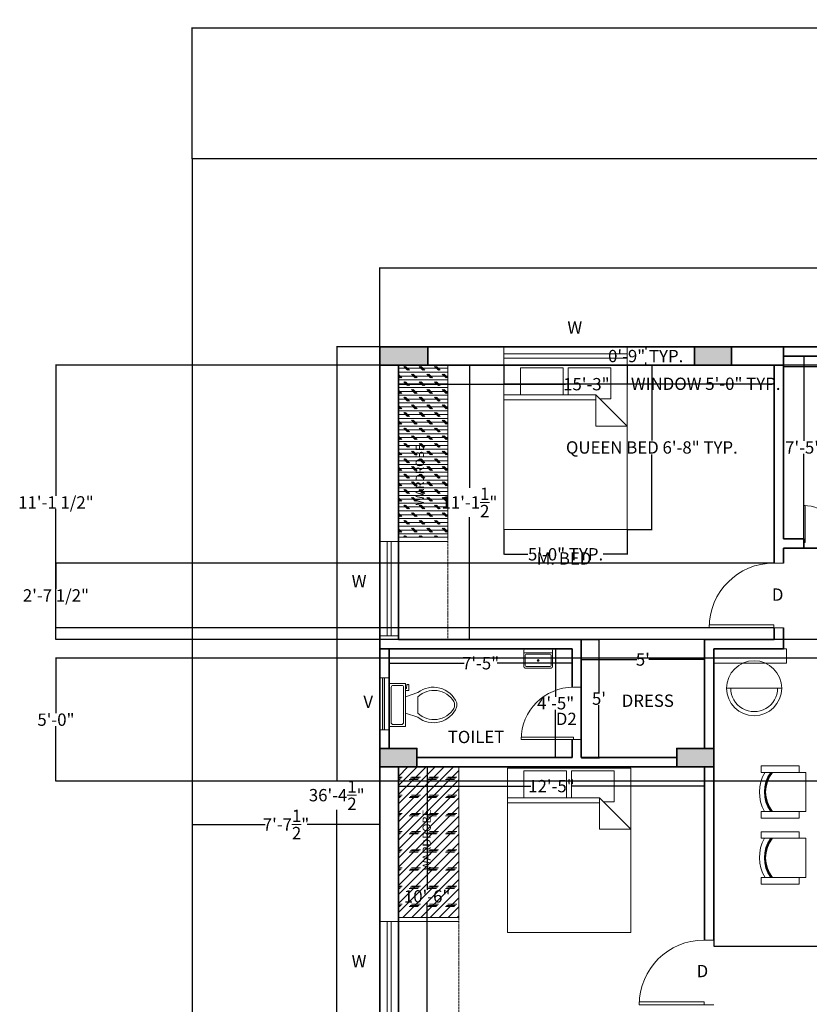
# Model space of a CAD drawing. Units: inches. Extents: x -2181 to 1225, y -80 to 4016.
# Tile 2 of 10: x -77 to 308, y 253 to 732. Entities that reach past the tile are written whole.
import ezdxf

# ---------------------------------------------------------------- set-up
doc = ezdxf.new("R2010")
doc.units = ezdxf.units.IN
doc.header["$MEASUREMENT"] = 0
doc.linetypes.add('ACAD_ISO02W100', pattern=[15, 12, -3])
for name, color, linetype, lineweight in [('A-ANNO-DIMS', 2, 'Continuous', 18), ('A-ANNO-TEXT', 7, 'Continuous', 18), ('A-AREA-IDEN', 7, 'Continuous', 18), ('A-COLS', 7, 'Continuous', 35), ('A-COLS-PATT', 252, 'Continuous', 13), ('A-DOOR', 3, 'Continuous', 18), ('A-FLOR-FIXT', 8, 'Continuous', 18), ('A-FURN', 30, 'Continuous', 18), ('A-GLAZ', 4, 'Continuous', 18), ('A-GLAZ-PATT', 4, 'Continuous', 13), ('A-MILL', 8, 'Continuous', 18), ('A-MILL-OVHD', 8, 'ACAD_ISO02W100', 13), ('A-MILL-PATT', 252, 'Continuous', 13), ('A-WALL', 7, 'Continuous', 35), ('A-WALL-OVHD', 7, 'ACAD_ISO02W100', 18), ('C-PROP', 7, 'Continuous', 30)]:
    doc.layers.add(name, color=color, linetype=linetype, lineweight=lineweight)
doc.styles.get("Standard").update_dxf_attribs({"font": 'arial.ttf'})
doc.dimstyles.get("Standard").update_dxf_attribs({"dimtxt": 6, "dimasz": 0.18, "dimexe": 0.18, "dimexo": 0.0625, "dimgap": 0.09, "dimtad": 0, "dimtih": 1, "dimtoh": 1, "dimdec": 4, "dimzin": 0, "dimdsep": 46, "dimlunit": 4, "dimtxsty": 'Standard', "dimcen": 0.09, "dimadec": 0, "dimazin": 0, "dimtfac": 1, "dimtdec": 4, "dimtofl": 0, "dimtmove": 0, "dimatfit": 3, "dimfxl": 1, "dimtolj": 1, "dimtzin": 0, "dimarcsym": 0})

# ---------------------------------------------------------------- blocks, each defined once
blk = doc.blocks.new('*U2')
for p, q in [((0, 0), (0, -6)), ((40, 0), (40, -6))]:
    blk.add_line(p, q)
blk.add_lwpolyline([(0, 0), (0, 40), (1.75, 40), (1.75, 0)], close=True)
blk.add_arc((0, 0), 40, 0, 90)
blk = doc.blocks.new('*U21')
for p, q in [((9.5, -6), (9.5, -2)), ((-10, -8.5), (-8, -8.5)), ((-10, -9.5), (-10, -8.5)), ((-7, -9.5), (-10, -9.5)), ((-8, -8.5), (-8, -8)), ((-7, -8), (-7, -9.5)), ((-4, -8), (-6, -14)), ((4, -8), (6, -14)), ((4, -14), (-4, -14))]:
    blk.add_line(p, q)
blk.add_lwpolyline([(10.5, -8), (10.5, 0), (-10.5, 0), (-10.5, -8)], close=True)
for points in [[(-9.5, -2), (-9.5, -6)], [(8.5, -1), (-8.5, -1)], [(-8.5, -7), (8.5, -7)]]:
    blk.add_lwpolyline(points)
for centre, radius, start, end in [((-8.62, -1.88), 0.884, 81.8699, 188.1301), ((8.62, -1.88), 0.884, 351.8699, 98.1301), ((-8.62, -6.12), 0.884, 171.8699, 278.1301), ((8.62, -6.12), 0.884, 261.8699, 8.1301), ((3.52, -21.58), 12.17, 141.4691, 247.9714), ((4.2, -21.82), 11.33, 136.3677, 238.9468), ((-3.52, -21.58), 12.17, 292.0284, 38.5307), ((-4.2, -21.82), 11.33, 301.053, 43.6321), ((0, -27.88), 4, 245.7318, 294.2682), ((0, -29), 4, 254.8605, 285.1395)]:
    blk.add_arc(centre, radius, start, end)
blk = doc.blocks.new('Bed - Queen')
for p, q in [((0, -80.00003), (0, 0)), ((0, 0), (59.99999, 0)), ((59.99999, 0), (59.99999, -80.00003)), ((7.99999, -1.2), (28.79998, -1.2)), ((7.99999, -14.4), (7.99999, -1.2)), ((28.79998, -1.2), (28.79998, -14.4)), ((31.19999, -1.2), (51.99999, -1.2)), ((31.19999, -14.4), (31.19999, -1.2)), ((51.99999, -1.2), (51.99999, -16.4)), ((0, -14.4), (44.8, -14.4)), ((44.8, -16.8), (0, -16.8)), ((59.99999, -29.6), (44.8, -14.4)), ((44.8, -14.4), (44.8, -29.6)), ((51.99999, -16.4), (46.79936, -16.4)), ((44.8, -29.6), (59.99999, -29.6)), ((59.99999, -80.00003), (0, -80.00003))]:
    blk.add_line(p, q)
blk = doc.blocks.new('*D23')
at = {"layer": 'A-ANNO-DIMS', "color": 0, "lineweight": -2, "transparency": 16777216}
for p, q in [((7.01, 340.55), (7.01, 340.66)), ((7.19, 340.48), (42.54, 340.48)), ((98.33, 340.48), (62.99, 340.48)), ((98.51, 340.55), (98.51, 340.66))]:
    blk.add_line(p, q, dxfattribs=at)
at = {"layer": 'A-ANNO-DIMS', "color": 0, "transparency": 16777216}
for points in [[(7.19, 340.51), (7.19, 340.45), (7.01, 340.48)], [(98.33, 340.51), (98.33, 340.45), (98.51, 340.48)]]:
    blk.add_solid(points, dxfattribs=at)
at = {"layer": 'Defpoints', "color": 0, "transparency": 16777216}
for p in [(7.01, 340.48), (98.51, 340.48), (98.51, 340.48)]:
    blk.add_point(p, dxfattribs=at)
at = {"layer": 'A-ANNO-DIMS', "color": 0, "transparency": 16777216, "insert": (52.76, 340.48), "char_height": 6, "attachment_point": 5}
blk.add_mtext('\\A1;7\'-7{\\H1x;\\S1/2;}"', dxfattribs=at)
blk = doc.blocks.new('*D26')
at = {"layer": 'A-ANNO-DIMS', "color": 0, "lineweight": -2, "transparency": 16777216}
for p, q in [((295.08, 568.48), (305, 568.48)), ((304.82, 568.3), (304.82, 527.13)), ((304.82, 479.66), (304.82, 520.84)), ((295.08, 479.48), (305, 479.48))]:
    blk.add_line(p, q, dxfattribs=at)
at = {"layer": 'A-ANNO-DIMS', "color": 0, "transparency": 16777216}
for points in [[(304.79, 568.3), (304.85, 568.3), (304.82, 568.48)], [(304.79, 479.66), (304.85, 479.66), (304.82, 479.48)]]:
    blk.add_solid(points, dxfattribs=at)
at = {"layer": 'Defpoints', "color": 0, "transparency": 16777216}
for p in [(295.01, 568.48), (295.01, 479.48), (304.82, 479.48)]:
    blk.add_point(p, dxfattribs=at)
at = {"layer": 'A-ANNO-DIMS', "color": 0, "transparency": 16777216, "insert": (304.82, 523.98), "char_height": 6, "attachment_point": 5}
blk.add_mtext('\\A1;7\'-5"', dxfattribs=at)
blk = doc.blocks.new('*D28')
at = {"layer": 'A-ANNO-DIMS', "color": 0, "lineweight": -2, "transparency": 16777216}
for p, q in [((295.01, 568.42), (295.01, 563.2)), ((355.01, 568.42), (355.01, 563.2)), ((295.19, 563.38), (322.16, 563.38)), ((354.83, 563.38), (327.87, 563.38))]:
    blk.add_line(p, q, dxfattribs=at)
at = {"layer": 'A-ANNO-DIMS', "color": 0, "transparency": 16777216}
for points in [[(295.19, 563.41), (295.19, 563.35), (295.01, 563.38)], [(354.83, 563.41), (354.83, 563.35), (355.01, 563.38)]]:
    blk.add_solid(points, dxfattribs=at)
at = {"layer": 'Defpoints', "color": 0, "transparency": 16777216}
for p in [(295.01, 568.48), (355.01, 568.48), (355.01, 563.38)]:
    blk.add_point(p, dxfattribs=at)
at = {"layer": 'A-ANNO-DIMS', "color": 0, "transparency": 16777216, "insert": (325.01, 563.38), "char_height": 6, "attachment_point": 5}
blk.add_mtext("\\A1;5'", dxfattribs=at)
blk = doc.blocks.new('*D30')
at = {"layer": 'A-ANNO-DIMS', "color": 0, "lineweight": -2, "transparency": 16777216}
for p, q in [((107.51, 563.92), (107.51, 554.61)), ((290.51, 563.92), (290.51, 554.61)), ((107.69, 554.79), (188.9, 554.79)), ((290.33, 554.79), (209.13, 554.79))]:
    blk.add_line(p, q, dxfattribs=at)
at = {"layer": 'A-ANNO-DIMS', "color": 0, "transparency": 16777216}
for points in [[(107.69, 554.82), (107.69, 554.76), (107.51, 554.79)], [(290.33, 554.82), (290.33, 554.76), (290.51, 554.79)]]:
    blk.add_solid(points, dxfattribs=at)
at = {"layer": 'Defpoints', "color": 0, "transparency": 16777216}
for p in [(107.51, 563.98), (290.51, 563.98), (290.51, 554.79)]:
    blk.add_point(p, dxfattribs=at)
at = {"layer": 'A-ANNO-DIMS', "color": 0, "transparency": 16777216, "insert": (199.01, 554.79), "char_height": 6, "attachment_point": 5}
blk.add_mtext('\\A1;15\'-3"', dxfattribs=at)
blk = doc.blocks.new('*D31')
at = {"layer": 'A-ANNO-DIMS', "color": 0, "lineweight": -2, "transparency": 16777216}
for p, q in [((107.58, 563.98), (142.27, 563.98)), ((142.09, 563.8), (142.09, 504.35)), ((142.09, 430.66), (142.09, 490.12)), ((107.58, 430.48), (142.27, 430.48))]:
    blk.add_line(p, q, dxfattribs=at)
at = {"layer": 'A-ANNO-DIMS', "color": 0, "transparency": 16777216}
for points in [[(142.06, 563.8), (142.12, 563.8), (142.09, 563.98)], [(142.06, 430.66), (142.12, 430.66), (142.09, 430.48)]]:
    blk.add_solid(points, dxfattribs=at)
at = {"layer": 'Defpoints', "color": 0, "transparency": 16777216}
for p in [(107.51, 563.98), (142.09, 563.98), (107.51, 430.48)]:
    blk.add_point(p, dxfattribs=at)
at = {"layer": 'A-ANNO-DIMS', "color": 0, "transparency": 16777216, "insert": (142.09, 497.23), "char_height": 6, "attachment_point": 5}
blk.add_mtext('\\A1;11\'-1{\\H1x;\\S1/2;}"', dxfattribs=at)
blk = doc.blocks.new('*D32')
at = {"layer": 'A-ANNO-DIMS', "color": 0, "lineweight": -2, "transparency": 16777216}
for p, q in [((103.01, 425.92), (103.01, 418.77)), ((192.01, 425.92), (192.01, 418.77)), ((103.19, 418.95), (139.47, 418.95)), ((191.83, 418.95), (155.55, 418.95))]:
    blk.add_line(p, q, dxfattribs=at)
at = {"layer": 'A-ANNO-DIMS', "color": 0, "transparency": 16777216}
for points in [[(103.19, 418.98), (103.19, 418.92), (103.01, 418.95)], [(191.83, 418.98), (191.83, 418.92), (192.01, 418.95)]]:
    blk.add_solid(points, dxfattribs=at)
at = {"layer": 'Defpoints', "color": 0, "transparency": 16777216}
for p in [(103.01, 425.98), (192.01, 425.98), (192.01, 418.95)]:
    blk.add_point(p, dxfattribs=at)
at = {"layer": 'A-ANNO-DIMS', "color": 0, "transparency": 16777216, "insert": (147.51, 418.95), "char_height": 6, "attachment_point": 5}
blk.add_mtext('\\A1;7\'-5"', dxfattribs=at)
blk = doc.blocks.new('*D33')
at = {"layer": 'A-ANNO-DIMS', "color": 0, "lineweight": -2, "transparency": 16777216}
for p, q in [((191.95, 425.98), (183.87, 425.98)), ((184.05, 425.8), (184.05, 402.63)), ((184.05, 373.16), (184.05, 396.34)), ((191.95, 372.98), (183.87, 372.98))]:
    blk.add_line(p, q, dxfattribs=at)
at = {"layer": 'A-ANNO-DIMS', "color": 0, "transparency": 16777216}
for points in [[(184.02, 425.8), (184.08, 425.8), (184.05, 425.98)], [(184.02, 373.16), (184.08, 373.16), (184.05, 372.98)]]:
    blk.add_solid(points, dxfattribs=at)
at = {"layer": 'Defpoints', "color": 0, "transparency": 16777216}
for p in [(184.05, 425.98), (192.01, 425.98), (192.01, 372.98)]:
    blk.add_point(p, dxfattribs=at)
at = {"layer": 'A-ANNO-DIMS', "color": 0, "transparency": 16777216, "insert": (184.05, 399.48), "char_height": 6, "attachment_point": 5}
blk.add_mtext('\\A1;4\'-5"', dxfattribs=at)
blk = doc.blocks.new('*D34')
at = {"layer": 'A-ANNO-DIMS', "color": 0, "lineweight": -2, "transparency": 16777216}
for p, q in [((196.51, 430.42), (196.51, 420.58)), ((256.51, 430.42), (256.51, 420.58)), ((196.69, 420.76), (223.66, 420.76)), ((256.33, 420.76), (229.37, 420.76))]:
    blk.add_line(p, q, dxfattribs=at)
at = {"layer": 'A-ANNO-DIMS', "color": 0, "transparency": 16777216}
for points in [[(196.69, 420.79), (196.69, 420.73), (196.51, 420.76)], [(256.33, 420.79), (256.33, 420.73), (256.51, 420.76)]]:
    blk.add_solid(points, dxfattribs=at)
at = {"layer": 'Defpoints', "color": 0, "transparency": 16777216}
for p in [(196.51, 430.48), (256.51, 430.48), (256.51, 420.76)]:
    blk.add_point(p, dxfattribs=at)
at = {"layer": 'A-ANNO-DIMS', "color": 0, "transparency": 16777216, "insert": (226.51, 420.76), "char_height": 6, "attachment_point": 5}
blk.add_mtext("\\A1;5'", dxfattribs=at)
blk = doc.blocks.new('*D35')
at = {"layer": 'A-ANNO-DIMS', "color": 0, "lineweight": -2, "transparency": 16777216}
for p, q in [((196.58, 430.48), (205.33, 430.48)), ((205.15, 430.3), (205.15, 404.88)), ((205.15, 373.16), (205.15, 398.59)), ((196.58, 372.98), (205.33, 372.98))]:
    blk.add_line(p, q, dxfattribs=at)
at = {"layer": 'A-ANNO-DIMS', "color": 0, "transparency": 16777216}
for points in [[(205.12, 430.3), (205.18, 430.3), (205.15, 430.48)], [(205.12, 373.16), (205.18, 373.16), (205.15, 372.98)]]:
    blk.add_solid(points, dxfattribs=at)
at = {"layer": 'Defpoints', "color": 0, "transparency": 16777216}
for p in [(196.51, 430.48), (205.15, 430.48), (196.51, 372.98)]:
    blk.add_point(p, dxfattribs=at)
at = {"layer": 'A-ANNO-DIMS', "color": 0, "transparency": 16777216, "insert": (205.15, 401.73), "char_height": 6, "attachment_point": 5}
blk.add_mtext("\\A1;5'", dxfattribs=at)
blk = doc.blocks.new('*D36')
at = {"layer": 'A-ANNO-DIMS', "color": 0, "lineweight": -2, "transparency": 16777216}
for p, q in [((107.51, 368.42), (107.51, 358.95)), ((256.51, 368.42), (256.51, 358.95)), ((107.69, 359.13), (171.9, 359.13)), ((256.33, 359.13), (192.13, 359.13))]:
    blk.add_line(p, q, dxfattribs=at)
at = {"layer": 'A-ANNO-DIMS', "color": 0, "transparency": 16777216}
for points in [[(107.69, 359.16), (107.69, 359.1), (107.51, 359.13)], [(256.33, 359.16), (256.33, 359.1), (256.51, 359.13)]]:
    blk.add_solid(points, dxfattribs=at)
at = {"layer": 'Defpoints', "color": 0, "transparency": 16777216}
for p in [(107.51, 368.48), (256.51, 368.48), (256.51, 359.13)]:
    blk.add_point(p, dxfattribs=at)
at = {"layer": 'A-ANNO-DIMS', "color": 0, "transparency": 16777216, "insert": (182.01, 359.13), "char_height": 6, "attachment_point": 5}
blk.add_mtext('\\A1;12\'-5"', dxfattribs=at)
blk = doc.blocks.new('*D37')
at = {"layer": 'A-ANNO-DIMS', "color": 0, "lineweight": -2, "transparency": 16777216}
for p, q in [((107.58, 368.48), (121.67, 368.48)), ((121.49, 368.3), (121.49, 308.64)), ((121.49, 242.66), (121.49, 302.33)), ((107.58, 242.48), (121.67, 242.48))]:
    blk.add_line(p, q, dxfattribs=at)
at = {"layer": 'A-ANNO-DIMS', "color": 0, "transparency": 16777216}
for points in [[(121.46, 368.3), (121.52, 368.3), (121.49, 368.48)], [(121.46, 242.66), (121.52, 242.66), (121.49, 242.48)]]:
    blk.add_solid(points, dxfattribs=at)
at = {"layer": 'Defpoints', "color": 0, "transparency": 16777216}
for p in [(107.51, 368.48), (121.49, 368.48), (107.51, 242.48)]:
    blk.add_point(p, dxfattribs=at)
at = {"layer": 'A-ANNO-DIMS', "color": 0, "transparency": 16777216, "insert": (121.49, 305.48), "char_height": 6, "attachment_point": 5}
blk.add_mtext('\\A1;10\'-6"', dxfattribs=at)
blk = doc.blocks.new('*D49')
at = {"layer": 'A-ANNO-DIMS', "color": 0, "lineweight": -2, "transparency": 16777216}
for p, q in [((261.01, 284.15), (261.01, 281.05)), ((261.19, 281.23), (335.37, 281.23)), ((419.33, 281.23), (345.16, 281.23)), ((419.51, 281.3), (419.51, 281.41))]:
    blk.add_line(p, q, dxfattribs=at)
at = {"layer": 'A-ANNO-DIMS', "color": 0, "transparency": 16777216}
for points in [[(261.19, 281.26), (261.19, 281.2), (261.01, 281.23)], [(419.33, 281.26), (419.33, 281.2), (419.51, 281.23)]]:
    blk.add_solid(points, dxfattribs=at)
at = {"layer": 'Defpoints', "color": 0, "transparency": 16777216}
for p in [(261.01, 284.21), (419.51, 281.23), (419.51, 281.23)]:
    blk.add_point(p, dxfattribs=at)
at = {"layer": 'A-ANNO-DIMS', "color": 0, "transparency": 16777216, "insert": (340.26, 281.23), "char_height": 6, "attachment_point": 5}
blk.add_mtext("\\A1;13'", dxfattribs=at)
blk = doc.blocks.new('*D70')
at = {"layer": 'A-ANNO-DIMS', "color": 0, "lineweight": -2, "transparency": 16777216}
for p, q in [((7.01, 664.55), (7.01, 728.44)), ((7.19, 728.26), (541.83, 728.26)), ((1086.83, 728.26), (552.2, 728.26)), ((1087.01, 664.55), (1087.01, 728.44))]:
    blk.add_line(p, q, dxfattribs=at)
at = {"layer": 'A-ANNO-DIMS', "color": 0, "transparency": 16777216}
for points in [[(7.19, 728.29), (7.19, 728.23), (7.01, 728.26)], [(1086.83, 728.29), (1086.83, 728.23), (1087.01, 728.26)]]:
    blk.add_solid(points, dxfattribs=at)
at = {"layer": 'Defpoints', "color": 0, "transparency": 16777216}
for p in [(1087.01, 728.26), (7.01, 664.48), (1087.01, 664.48)]:
    blk.add_point(p, dxfattribs=at)
at = {"layer": 'A-ANNO-DIMS', "color": 0, "transparency": 16777216, "insert": (547.01, 728.26), "char_height": 6, "attachment_point": 5}
blk.add_mtext("\\A1;90'", dxfattribs=at)
blk = doc.blocks.new('Sink-single - 30 in top')
blk.add_line((-15, -3.999996), (15, -3.999996))
for points in [[(-13.5, 0), (13.5, 0)], [(-15, -18.499996), (-15, -1.5)], [(-13.5, -17.499996), (-13.5, -6.499996)], [(-12.5, -5.499996), (12.5, -5.499996)], [(13.5, -6.499996), (13.5, -17.499996)], [(15, -1.5), (15, -18.499996)], [(13.5, -19.999996), (-13.5, -19.999996)], [(12.5, -18.499996), (-12.5, -18.499996)]]:
    blk.add_lwpolyline(points)
for radius in [1, 0.5]:
    blk.add_circle((0, -11.999996), radius)
for centre, radius, start, end in [((-13.5, -1.5), 1.5, 90, 180), ((-12.5, -6.499996), 1, 90, 180), ((12.5, -6.499996), 1, 0, 90), ((13.5, -1.5), 1.5, 0, 90), ((-13.5, -18.499996), 1.5, 180, 270), ((-12.5, -17.499996), 1, 180, 270), ((12.5, -17.499996), 1, 270, 0), ((13.5, -18.499996), 1.5, 270, 0)]:
    blk.add_arc(centre, radius, start, end)
blk = doc.blocks.new('*D71')
at = {"layer": 'A-ANNO-DIMS', "color": 0, "lineweight": -2, "transparency": 16777216}
for p, q in [((98.51, 573.05), (98.51, 611.58)), ((98.69, 611.4), (536.64, 611.4)), ((995.33, 611.4), (557.39, 611.4)), ((995.51, 573.05), (995.51, 611.58))]:
    blk.add_line(p, q, dxfattribs=at)
at = {"layer": 'A-ANNO-DIMS', "color": 0, "transparency": 16777216}
for points in [[(98.69, 611.43), (98.69, 611.37), (98.51, 611.4)], [(995.33, 611.43), (995.33, 611.37), (995.51, 611.4)]]:
    blk.add_solid(points, dxfattribs=at)
at = {"layer": 'Defpoints', "color": 0, "transparency": 16777216}
for p in [(995.51, 611.4), (98.51, 572.98), (995.51, 572.98)]:
    blk.add_point(p, dxfattribs=at)
at = {"layer": 'A-ANNO-DIMS', "color": 0, "transparency": 16777216, "insert": (547.01, 611.4), "char_height": 6, "attachment_point": 5}
blk.add_mtext('\\A1;74\'-9"', dxfattribs=at)
blk = doc.blocks.new('*D72')
at = {"layer": 'A-ANNO-DIMS', "color": 0, "lineweight": -2, "transparency": 16777216}
for p, q in [((98.45, 572.98), (77.28, 572.98)), ((77.46, 572.8), (77.46, 361.9)), ((77.46, 136.66), (77.46, 347.57)), ((98.45, 136.48), (77.28, 136.48))]:
    blk.add_line(p, q, dxfattribs=at)
at = {"layer": 'A-ANNO-DIMS', "color": 0, "transparency": 16777216}
for points in [[(77.43, 572.8), (77.49, 572.8), (77.46, 572.98)], [(77.43, 136.66), (77.49, 136.66), (77.46, 136.48)]]:
    blk.add_solid(points, dxfattribs=at)
at = {"layer": 'Defpoints', "color": 0, "transparency": 16777216}
for p in [(77.46, 572.98), (98.51, 572.98), (98.51, 136.48)]:
    blk.add_point(p, dxfattribs=at)
at = {"layer": 'A-ANNO-DIMS', "color": 0, "transparency": 16777216, "insert": (77.46, 354.73), "char_height": 6, "attachment_point": 5}
blk.add_mtext('\\A1;36\'-4{\\H1x;\\S1/2;}"', dxfattribs=at)
blk = doc.blocks.new('DINING-CHAIR-SIDE')
for p, q in [((0.79, 22.26), (0.79, 25.47)), ((19.33, 22.26), (19.33, 25.47)), ((0.79, 0), (0.79, 3.21)), ((19.33, 3.21), (19.33, 0))]:
    blk.add_line(p, q)
for points in [[(0.79, 25.47), (19.33, 25.47)], [(0.79, 22.26), (22.53, 22.26), (22.53, 3.21), (0.79, 3.21)], [(19.33, 0), (0.79, 0)]]:
    blk.add_lwpolyline(points)
for centre, radius, start, end in [((19.12, 12.45), 19.13, 149.1418, 208.8973), ((18.29, 12.73), 15.92, 143.2428, 216.7572), ((18.29, 12.73), 15.6, 142.3578, 217.6422), ((18.29, 12.73), 15.28, 141.4242, 218.5758)]:
    blk.add_arc(centre, radius, start, end)
blk = doc.blocks.new('BASIN-ROUND')
blk.add_line((13.41, 0), (13.41, 26.83))
blk.add_circle((13.41, 13.41), 13.41)
blk.add_arc((13.41, 13.41), 11.41, 270, 90)
blk = doc.blocks.new('COL-18X9')
blk.add_lwpolyline([(0, 9), (18, 9), (18, 0), (0, 0)], close=True)
blk = doc.blocks.new('WIN-60')
for p, q in [((0, 0), (0, 9)), ((0, 5.5), (60, 5.5)), ((60, 0), (60, 9)), ((0, 3.5), (60, 3.5))]:
    blk.add_line(p, q)
blk = doc.blocks.new('*D96')
at = {"layer": 'A-ANNO-DIMS', "color": 0, "lineweight": -2, "transparency": 16777216}
for p, q in [((218.95, 563.98), (231.07, 563.98)), ((230.89, 563.8), (230.89, 527.36)), ((230.89, 484.16), (230.89, 520.61)), ((218.95, 483.98), (231.07, 483.98))]:
    blk.add_line(p, q, dxfattribs=at)
at = {"layer": 'A-ANNO-DIMS', "color": 0, "transparency": 16777216}
for points in [[(230.86, 563.8), (230.92, 563.8), (230.89, 563.98)], [(230.86, 484.16), (230.92, 484.16), (230.89, 483.98)]]:
    blk.add_solid(points, dxfattribs=at)
at = {"layer": 'Defpoints', "color": 0, "transparency": 16777216}
for p in [(218.89, 563.98), (230.89, 563.98), (218.89, 483.98)]:
    blk.add_point(p, dxfattribs=at)
at = {"layer": 'A-ANNO-DIMS', "color": 0, "transparency": 16777216, "insert": (230.89, 523.98), "char_height": 6, "attachment_point": 5}
blk.add_mtext('\\A1;QUEEN BED 6\'-8" TYP.', dxfattribs=at)
blk = doc.blocks.new('*D97')
at = {"layer": 'A-ANNO-DIMS', "color": 0, "lineweight": -2, "transparency": 16777216}
for p, q in [((158.89, 483.92), (158.89, 471.8)), ((218.89, 483.92), (218.89, 471.8)), ((159.07, 471.98), (170.51, 471.98)), ((218.71, 471.98), (207.26, 471.98))]:
    blk.add_line(p, q, dxfattribs=at)
at = {"layer": 'A-ANNO-DIMS', "color": 0, "transparency": 16777216}
for points in [[(159.07, 472.01), (159.07, 471.95), (158.89, 471.98)], [(218.71, 472.01), (218.71, 471.95), (218.89, 471.98)]]:
    blk.add_solid(points, dxfattribs=at)
at = {"layer": 'Defpoints', "color": 0, "transparency": 16777216}
for p in [(158.89, 483.98), (218.89, 483.98), (218.89, 471.98)]:
    blk.add_point(p, dxfattribs=at)
at = {"layer": 'A-ANNO-DIMS', "color": 0, "transparency": 16777216, "insert": (188.89, 471.98), "char_height": 6, "attachment_point": 5}
blk.add_mtext('\\A1;5\'-0" TYP.', dxfattribs=at)
blk = doc.blocks.new('*D122')
at = {"layer": 'A-ANNO-DIMS', "color": 0, "lineweight": -2, "transparency": 16777216}
for p, q in [((158.89, 563.92), (158.89, 554.8)), ((218.89, 563.92), (218.89, 554.8)), ((159.07, 554.98), (218.71, 554.98)), ((218.89, 554.98), (219.07, 554.98))]:
    blk.add_line(p, q, dxfattribs=at)
at = {"layer": 'A-ANNO-DIMS', "color": 0, "transparency": 16777216}
for points in [[(159.07, 555.01), (159.07, 554.95), (158.89, 554.98)], [(218.71, 555.01), (218.71, 554.95), (218.89, 554.98)]]:
    blk.add_solid(points, dxfattribs=at)
at = {"layer": 'Defpoints', "color": 0, "transparency": 16777216}
for p in [(158.89, 563.98), (218.89, 563.98), (218.89, 554.98)]:
    blk.add_point(p, dxfattribs=at)
at = {"layer": 'A-ANNO-DIMS', "color": 0, "transparency": 16777216, "insert": (257.12, 554.98), "char_height": 6, "attachment_point": 5}
blk.add_mtext('\\A1;WINDOW 5\'-0" TYP.', dxfattribs=at)
blk = doc.blocks.new('*D123')
at = {"layer": 'A-ANNO-DIMS', "color": 0, "lineweight": -2, "transparency": 16777216}
for p, q in [((218.95, 572.98), (228.07, 572.98)), ((227.89, 572.8), (227.89, 571.64)), ((218.95, 563.98), (228.07, 563.98)), ((227.89, 564.16), (227.89, 565.33))]:
    blk.add_line(p, q, dxfattribs=at)
at = {"layer": 'A-ANNO-DIMS', "color": 0, "transparency": 16777216}
for points in [[(227.86, 572.8), (227.92, 572.8), (227.89, 572.98)], [(227.86, 564.16), (227.92, 564.16), (227.89, 563.98)]]:
    blk.add_solid(points, dxfattribs=at)
at = {"layer": 'Defpoints', "color": 0, "transparency": 16777216}
for p in [(218.89, 572.98), (227.89, 572.98), (218.89, 563.98)]:
    blk.add_point(p, dxfattribs=at)
at = {"layer": 'A-ANNO-DIMS', "color": 0, "transparency": 16777216, "insert": (227.89, 568.48), "char_height": 6, "attachment_point": 5}
blk.add_mtext('\\A1;0\'-9" TYP.', dxfattribs=at)
blk = doc.blocks.new('*D130')
at = {"layer": 'A-ANNO-DIMS', "color": 0, "lineweight": -2, "transparency": 16777216}
for p, q in [((512.45, 421.48), (-59.44, 421.48)), ((-59.26, 421.3), (-59.26, 394.64)), ((-59.26, 361.66), (-59.26, 388.33)), ((512.45, 361.48), (-59.44, 361.48))]:
    blk.add_line(p, q, dxfattribs=at)
at = {"layer": 'A-ANNO-DIMS', "color": 0, "transparency": 16777216}
for points in [[(-59.29, 421.3), (-59.23, 421.3), (-59.26, 421.48)], [(-59.29, 361.66), (-59.23, 361.66), (-59.26, 361.48)]]:
    blk.add_solid(points, dxfattribs=at)
at = {"layer": 'Defpoints', "color": 0, "transparency": 16777216}
for p in [(512.51, 421.48), (-59.26, 361.48), (512.51, 361.48)]:
    blk.add_point(p, dxfattribs=at)
at = {"layer": 'A-ANNO-DIMS', "color": 0, "transparency": 16777216, "insert": (-59.26, 391.48), "char_height": 6, "attachment_point": 5}
blk.add_mtext('\\A1;5\'-0"', dxfattribs=at)
blk = doc.blocks.new('*D131')
at = {"layer": 'A-ANNO-DIMS', "color": 0, "lineweight": -2, "transparency": 16777216}
for p, q in [((976.64, 563.98), (-59.44, 563.98)), ((-59.26, 563.8), (-59.26, 500.43)), ((-59.26, 430.66), (-59.26, 494.04)), ((977.45, 430.48), (-59.44, 430.48))]:
    blk.add_line(p, q, dxfattribs=at)
at = {"layer": 'A-ANNO-DIMS', "color": 0, "transparency": 16777216}
for points in [[(-59.29, 563.8), (-59.23, 563.8), (-59.26, 563.98)], [(-59.29, 430.66), (-59.23, 430.66), (-59.26, 430.48)]]:
    blk.add_solid(points, dxfattribs=at)
at = {"layer": 'Defpoints', "color": 0, "transparency": 16777216}
for p in [(976.7, 563.98), (-59.26, 430.48), (977.51, 430.48)]:
    blk.add_point(p, dxfattribs=at)
at = {"layer": 'A-ANNO-DIMS', "color": 0, "transparency": 16777216, "insert": (-59.26, 497.23), "char_height": 6, "attachment_point": 5}
blk.add_mtext('\\A1;11\'-1 1/2"', dxfattribs=at)
blk = doc.blocks.new('*D132')
at = {"layer": 'A-ANNO-DIMS', "color": 0, "lineweight": -2, "transparency": 16777216}
for p, q in [((290.45, 467.72), (-59.44, 467.72)), ((-59.26, 467.54), (-59.26, 455.16)), ((-59.26, 436.39), (-59.26, 448.77)), ((290.45, 436.21), (-59.44, 436.21))]:
    blk.add_line(p, q, dxfattribs=at)
at = {"layer": 'A-ANNO-DIMS', "color": 0, "transparency": 16777216}
for points in [[(-59.29, 467.54), (-59.23, 467.54), (-59.26, 467.72)], [(-59.29, 436.39), (-59.23, 436.39), (-59.26, 436.21)]]:
    blk.add_solid(points, dxfattribs=at)
at = {"layer": 'Defpoints', "color": 0, "transparency": 16777216}
for p in [(-59.26, 467.72), (290.51, 467.72), (290.51, 436.21)]:
    blk.add_point(p, dxfattribs=at)
at = {"layer": 'A-ANNO-DIMS', "color": 0, "transparency": 16777216, "insert": (-59.26, 451.96), "char_height": 6, "attachment_point": 5}
blk.add_mtext('\\A1;2\'-7 1/2"', dxfattribs=at)

msp = doc.modelspace()

# ---------------------------------------------------------------- hatches: boundary and pattern name
at = {"layer": 'A-COLS-PATT'}
h = msp.add_hatch(color=256, dxfattribs=at)
h.dxf.hatch_style = 1
h.paths.add_polyline_path([(437.51461, 572.98479), (419.51461, 572.98479), (419.51461, 563.98479), (437.51461, 563.98479)])
h.paths.add_polyline_path([(269.65161, 572.98479), (251.65161, 572.98479), (251.65161, 563.98479), (269.65161, 563.98479)])
h.paths.add_polyline_path([(121.82546, 572.98479), (103.01461, 572.98479), (98.51461, 572.98479), (98.51461, 563.98479), (116.51461, 563.98479), (121.82546, 563.98479)])
h.paths.add_polyline_path([(116.51461, 377.48479), (98.51461, 377.48479), (98.51461, 368.48479), (116.51461, 368.48479)])
h.paths.add_polyline_path([(261.01461, 377.48479), (243.01461, 377.48479), (243.01461, 368.48479), (261.01461, 368.48479)])
at = {"layer": 'A-GLAZ-PATT'}
h = msp.add_hatch(color=256, dxfattribs=at)
h.dxf.hatch_style = 1
h.paths.add_polyline_path([(100.76461, 411.89133), (99.76461, 411.89133), (99.76461, 386.51661), (100.76461, 386.51661)])
h.paths.add_polyline_path([(341.43431, 571.73479), (317.43431, 571.73479), (317.43431, 570.73479), (341.43431, 570.73479)])
h.paths.add_polyline_path([(399.07838, 571.73479), (375.07838, 571.73479), (375.07838, 570.73479), (399.07838, 570.73479)])
at = {"layer": 'A-MILL-PATT'}
h = msp.add_hatch(dxfattribs=at)
h.set_pattern_fill('CORK', color=256, scale=15)
h.set_pattern_definition([(0, (-759, -3e-13), (0, 1.875), []), (135, (-758.0625, -0.9375), (-3.75, -3.75), [2.65165, -2.65165]), (135, (-757.594, -0.9375), (-3.75, -3.75), [2.65165, -2.65165]), (135, (-757.125, -0.9375), (-3.75, -3.75), [2.65165, -2.65165])])
h.paths.add_polyline_path([(107.51461, 480.27202), (131.51461, 480.27202), (131.51461, 563.98479), (107.51461, 563.98479)])
h = msp.add_hatch(dxfattribs=at)
h.set_pattern_fill('CORK', color=256, scale=25, angle=45)
h.set_pattern_definition([(45, (0, 0), (-2.209709, 2.209709), []), (180, (2.21, 0), (-9e-16, -8.83883), [4.41942, -4.41942]), (180, (2.762, 0.552), (-9e-16, -8.83883), [4.41942, -4.41942]), (180, (3.315, 1.105), (-9e-16, -8.83883), [4.41942, -4.41942])])
h.paths.add_polyline_path([(136.8586, 368.48479), (107.51461, 368.48479), (107.51461, 295.2354), (136.8586, 295.2354)])

# ---------------------------------------------------------------- linework, layer by layer
at = {"layer": 'A-COLS'}
for points in [[(116.51461, 563.98479), (98.51461, 563.98479), (98.51461, 572.98479), (116.51461, 572.98479)], [(103.01461, 572.98479), (121.82546, 572.98479), (121.82546, 563.98479), (103.01461, 563.98479)]]:
    msp.add_lwpolyline(points, dxfattribs=at)
at = {"layer": 'A-GLAZ'}
for p, q in [((131.51461, 478.27202), (98.51461, 478.27202)), ((102.01461, 432.27202), (102.01461, 478.27202)), ((104.01461, 432.27202), (104.01461, 478.27202)), ((107.51461, 432.27202), (98.51461, 432.27202)), ((103.01461, 411.89133), (98.51461, 411.89133)), ((99.76461, 386.51661), (99.76461, 411.89133)), ((100.76461, 386.51661), (100.76461, 411.89133)), ((98.51461, 386.51661), (103.01461, 386.51661)), ((136.8586, 293.2354), (98.51461, 293.2354)), ((102.01461, 247.37629), (102.01461, 293.2354)), ((104.01461, 247.37629), (104.01461, 293.2354))]:
    msp.add_line(p, q, dxfattribs=at)
at = {"layer": 'A-MILL'}
for p, q in [((107.51461, 563.98479), (131.51461, 563.98479)), ((131.51461, 563.98479), (131.51461, 480.27202)), ((107.51461, 480.27202), (131.51461, 480.27202))]:
    msp.add_line(p, q, dxfattribs=at)
for points in [[(261.01461, 425.98479), (296.52633, 425.98479), (296.52633, 419.0568), (261.01461, 419.0568)], [(107.51461, 368.48479), (136.8586, 368.48479), (136.8586, 295.2354), (107.51461, 295.2354)]]:
    msp.add_lwpolyline(points, close=True, dxfattribs=at)
at = {"layer": 'A-MILL-OVHD', "ltscale": 0.1}
for p, q in [((131.51461, 480.27202), (131.51461, 430.48479)), ((136.8586, 295.2354), (136.8586, 242.48479))]:
    msp.add_line(p, q, dxfattribs=at)
at = {"layer": 'A-WALL'}
for p, q in [((304.81567, 479.48479), (304.81567, 474.98479)), ((196.51461, 430.48479), (107.51461, 430.48479)), ((196.51461, 430.48479), (196.51461, 407.25481)), ((256.51461, 430.48479), (256.51461, 377.48479)), ((256.51461, 430.48479), (290.51461, 430.48479)), ((107.51461, 425.98479), (103.01461, 425.98479)), ((103.01461, 425.98479), (103.01461, 377.48479)), ((192.01461, 425.98479), (192.01461, 407.24561)), ((261.01461, 425.98479), (261.01461, 284.21083)), ((196.51461, 407.25481), (196.51461, 372.98479)), ((192.01461, 381.81654), (192.01461, 372.98479)), ((107.51461, 368.48479), (98.51461, 368.48479)), ((256.51461, 368.48479), (256.51461, 284.21083)), ((98.51461, 295.2354), (98.51461, 295.2354))]:
    msp.add_line(p, q, dxfattribs=at)
for points in [[(587.51461, 572.98479), (98.51461, 572.98479), (98.51461, 136.48479)], [(295.01461, 572.98479), (295.01461, 479.48479)], [(355.01461, 568.48479), (295.01461, 568.48479)], [(107.51461, 563.98479), (107.51461, 430.48479)], [(290.51461, 563.98479), (107.51461, 563.98479)], [(107.51461, 459.32103), (107.51461, 563.98479)], [(295.01461, 563.98479), (107.51461, 563.98479), (107.51461, 434.98479)], [(290.51461, 563.98479), (290.51461, 467.71596)], [(304.81567, 479.48479), (295.01461, 479.48479)], [(359.51461, 474.98479), (295.01461, 474.98479)], [(295.01461, 474.98479), (295.01461, 467.71596)], [(290.51461, 436.21069), (290.51461, 430.48479)], [(295.01461, 436.21069), (295.01461, 425.98479)], [(98.51461, 425.98479), (98.51461, 425.98479), (103.01461, 425.98479)], [(192.01461, 425.98479), (107.51461, 425.98479)], [(295.01461, 425.98479), (261.01461, 425.98479)], [(192.01461, 372.98479), (116.51461, 372.98479)], [(243.01461, 372.98479), (196.51461, 372.98479)], [(261.01461, 368.48479), (103.01461, 368.48479)], [(107.51461, 368.48479), (107.51461, 242.48479)]]:
    msp.add_lwpolyline(points, dxfattribs=at)
at = {"layer": 'A-WALL-OVHD', "ltscale": 0.1}
msp.add_lwpolyline([(256.51461, 430.48479), (196.51461, 430.48479)], dxfattribs=at)
at = {"layer": 'C-PROP'}
msp.add_lwpolyline([(1087.01461, 16.48479), (1087.01461, 664.48479), (7.01461, 664.48479), (7.01461, 16.48479)], dxfattribs=at)

# ---------------------------------------------------------------- block references
at = {"layer": 'A-COLS', "extrusion": (0, 0, -1), "zscale": -1, "rotation": 180}
for p in [(-251.65199, 572.98457), (-98.515, 377.48457), (-243.015, 377.48457)]:
    msp.add_blockref('COL-18X9', p, dxfattribs=at)
at = {"layer": 'A-DOOR', "xscale": 0.4503069535887608, "yscale": 0.4503069535887608, "zscale": 0.4503069535887608}
msp.add_blockref('*U2', (304.81567, 477.68663), dxfattribs=at)
at = {"layer": 'A-DOOR', "rotation": 90.00000000000003}
for p, xscale, yscale, zscale in [((290.28882, 436.21069), 0.7876317507006553, 0.7876317507006553, 0.7876317507006553), ((192.69887, 381.81654), 0.6359567768907052, 0.6359567768907052, 0.6359567768907052), ((256.28882, 252.70556), 0.7876317507006553, 0.7876317507006553, 0.7876317507006553)]:
    msp.add_blockref('*U2', p, dxfattribs=dict(at, xscale=xscale, yscale=yscale, zscale=zscale))
at = {"layer": 'A-FLOR-FIXT', "xscale": -0.4649637902209482, "yscale": 0.4649637902209482, "zscale": 0.4649637902209482}
msp.add_blockref('Sink-single - 30 in top', (175.51948, 425.92367), dxfattribs=at)
at = {"layer": 'A-FLOR-FIXT', "extrusion": (0, 0, -1), "zscale": -1, "rotation": 269.9999999999998}
msp.add_blockref('BASIN-ROUND', (-294.11752, 420.19668), dxfattribs=at)
at = {"layer": 'A-FLOR-FIXT', "xscale": -1, "rotation": 89.90827745497215}
msp.add_blockref('*U21', (102.99609, 398.66447), dxfattribs=at)
at = {"layer": 'A-FURN'}
for name, p in [('Bed - Queen', (158.88661, 563.98479)), ('DINING-CHAIR-SIDE', (283.2957, 343.58385)), ('Bed - Queen', (160.60741, 367.81097))]:
    msp.add_blockref(name, p, dxfattribs=at)
at = {"layer": 'A-FURN', "extrusion": (0, 0, -1), "zscale": -1, "rotation": 180}
msp.add_blockref('DINING-CHAIR-SIDE', (-283.2957, 336.94792), dxfattribs=at)
at = {"layer": 'A-GLAZ'}
msp.add_blockref('WIN-60', (158.887, 563.985), dxfattribs=at)

# ---------------------------------------------------------------- texts
at = {"layer": 'A-ANNO-TEXT', "char_height": 6, "attachment_point": 1}
for s, insert in [('W', (189.77524, 585.35008)), ('W', (84.74546, 461.85968)), ('D', (289.34202, 455.34612)), ('V', (90.43216, 403.17621)), ('D2', (184.13309, 394.8592)), ('W', (84.72585, 276.88707)), ('D', (252.69364, 272.11988))]:
    msp.add_mtext_dynamic_manual_height_columns(s, width=291.4178321, gutter_width=1, heights=[0], dxfattribs=dict(at, insert=insert))
at = {"layer": 'A-ANNO-TEXT', "char_height": 4, "attachment_point": 1, "rotation": 90}
for insert in [(115.89948, 495.73488), (119.2704, 318.09448)]:
    msp.add_mtext_dynamic_manual_height_columns('WARDROBE', width=13.1749235, gutter_width=1, heights=[0], dxfattribs=dict(at, insert=insert))
at = {"layer": 'A-AREA-IDEN', "char_height": 6, "attachment_point": 1}
for s, insert in [('M. BED', (174.8517, 472.96742)), ('DRESS', (216.22499, 403.71747)), ('TOILET', (131.51802, 386.058))]:
    msp.add_mtext_dynamic_manual_height_columns(s, width=291.4178321, gutter_width=1, heights=[0], dxfattribs=dict(at, insert=insert))

# ---------------------------------------------------------------- dimensions: what is measured, and where the dimension line sits
at = {"layer": 'A-ANNO-DIMS'}
for base, p1, p2, picture, middle in [((1087.01461, 728.26231), (7.01461, 664.48479), (1087.01461, 664.48479), '*D70', (547.01461, 728.26231)), ((995.51461, 611.40365), (98.51461, 572.98479), (995.51461, 572.98479), '*D71', (547.01461, 611.40365)), ((355.01461, 563.38158), (295.01461, 568.48479), (355.01461, 568.48479), '*D28', (325.01461, 563.38158)), ((290.51461, 554.78898), (107.51461, 563.98479), (290.51461, 563.98479), '*D30', (199.01461, 554.78898)), ((256.51461, 420.75538), (196.51461, 430.48479), (256.51461, 430.48479), '*D34', (226.51461, 420.75538)), ((192.01461, 418.94683), (103.01461, 425.98479), (192.01461, 425.98479), '*D32', (147.51461, 418.94683)), ((256.51461, 359.12646), (107.51461, 368.48479), (256.51461, 368.48479), '*D36', (182.01461, 359.12646)), ((98.51461, 340.48479), (7.01461, 340.48479), (98.51461, 340.48479), '*D23', (52.76461, 340.48479))]:
    dim = msp.add_linear_dim(base=base, p1=p1, p2=p2, dimstyle='Standard', override={"dimclrd": 0, "dimclre": 0, "dimclrt": 0}, dxfattribs=at)
    dim.commit()
    dim.dimension.update_dxf_attribs({"geometry": picture, "text_midpoint": middle})
for base, p1, p2, text, override, picture, middle in [((227.8866, 572.98479), (218.8866, 563.98479), (218.8866, 572.98479), '<> TYP.', {"dimdec": 1, "dimlfac": 1, "dimrnd": 0, "dimzin": 1, "dimdsep": 46, "dimlunit": 4, "dimfrac": 2}, '*D123', (227.8866, 568.48479)), ((230.8866, 563.98479), (218.8866, 483.98476), (218.8866, 563.98479), 'QUEEN BED <> TYP.', {"dimdec": 1, "dimlfac": 1, "dimrnd": 0, "dimzin": 1, "dimdsep": 46, "dimlunit": 4, "dimfrac": 2}, '*D96', (230.8866, 523.98477)), ((205.15171, 430.48479), (196.51461, 372.98479), (196.51461, 430.48479), "5'", {"dimclrd": 0, "dimclre": 0, "dimclrt": 0}, '*D35', (205.15171, 401.73479))]:
    dim = msp.add_linear_dim(base=base, p1=p1, p2=p2, angle=90, text=text, dimstyle='Standard', override=override, dxfattribs=at)
    dim.commit()
    dim.dimension.update_dxf_attribs({"geometry": picture, "text_midpoint": middle})
for base, p1, p2, override, picture, middle in [((77.46081, 572.98479), (98.51461, 136.48479), (98.51461, 572.98479), {"dimclrd": 0, "dimclre": 0, "dimclrt": 0}, '*D72', (77.46081, 354.73479)), ((304.81567, 479.48479), (295.01461, 568.48479), (295.01461, 479.48479), {"dimclrd": 0, "dimclre": 0, "dimclrt": 0}, '*D26', (304.81567, 523.98479)), ((-59.2566, 430.48478), (976.70377, 563.98478), (977.51461, 430.48478), {"dimdec": 1, "dimlfac": 1, "dimrnd": 0, "dimzin": 1, "dimdsep": 46, "dimlunit": 4, "dimfrac": 2}, '*D131', (-59.2566, 497.23478)), ((142.08883, 563.98479), (107.51461, 430.48479), (107.51461, 563.98479), {"dimclrd": 0, "dimclre": 0, "dimclrt": 0}, '*D31', (142.08883, 497.23479)), ((-59.2566, 467.71596), (290.51461, 436.21069), (290.51461, 467.71596), {"dimdec": 1, "dimlfac": 1, "dimrnd": 0, "dimzin": 1, "dimdsep": 46, "dimlunit": 4, "dimfrac": 2}, '*D132', (-59.2566, 451.96332)), ((184.04903, 425.98479), (192.01461, 372.98479), (192.01461, 425.98479), {"dimclrd": 0, "dimclre": 0, "dimclrt": 0}, '*D33', (184.04903, 399.48479)), ((-59.2566, 361.48478), (512.51461, 421.48478), (512.51461, 361.48478), {"dimdec": 1, "dimlfac": 1, "dimrnd": 0, "dimzin": 1, "dimdsep": 46, "dimlunit": 4, "dimfrac": 2}, '*D130', (-59.2566, 391.48478)), ((121.48843, 368.48479), (107.51461, 242.48479), (107.51461, 368.48479), {"dimclrd": 0, "dimclre": 0, "dimclrt": 0}, '*D37', (121.48843, 305.48479))]:
    dim = msp.add_linear_dim(base=base, p1=p1, p2=p2, angle=90, dimstyle='Standard', override=override, dxfattribs=at)
    dim.commit()
    dim.dimension.update_dxf_attribs({"geometry": picture, "text_midpoint": middle})
for base, p1, p2, text, override, picture, middle in [((218.8866, 554.98479), (158.88661, 563.98479), (218.8866, 563.98479), 'WINDOW <> TYP.', {"dimdec": 1, "dimlfac": 1, "dimrnd": 0, "dimzin": 1, "dimdsep": 46, "dimlunit": 4, "dimfrac": 2}, '*D122', (257.11908, 554.98479)), ((218.8866, 471.98475), (158.88661, 483.98476), (218.8866, 483.98476), '<> TYP.', {"dimdec": 1, "dimlfac": 1, "dimrnd": 0, "dimzin": 1, "dimdsep": 46, "dimlunit": 4, "dimfrac": 2}, '*D97', (188.8866, 471.98475)), ((419.51461, 281.23479), (261.01461, 284.21083), (419.51461, 281.23479), "13'", {"dimclrd": 0, "dimclre": 0, "dimclrt": 0}, '*D49', (340.26461, 281.23479))]:
    dim = msp.add_linear_dim(base=base, p1=p1, p2=p2, text=text, dimstyle='Standard', override=override, dxfattribs=at)
    dim.commit()
    dim.dimension.update_dxf_attribs({"geometry": picture, "text_midpoint": middle})

doc.saveas('drawing.dxf')
